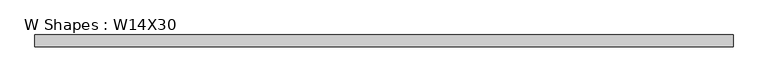
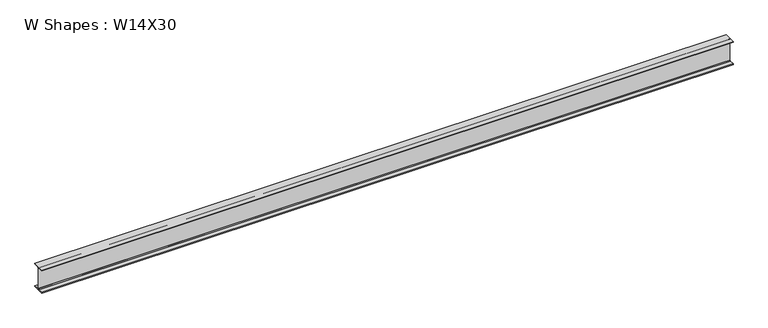
"""IFC4 building model written with IfcOpenShell, lengths in millimetres: beam geometry, W Shapes : W14X30."""

from ifc_helpers import new_model, si_unit, point, frame, frame_2d, origin, place, context, project, spatial, polyline, circle_curve, trimmed, segment, composite_curve, outline, extrude, source, transform, mapped, element, save


def w_shapes_w14x30_541e514d(model_context):
    return source(origin(), model_context, "Body", "SweptSolid", [
        extrude(outline(composite_curve([segment(polyline([(85.471, -165.481), (85.471, -175.26), (-85.471, -175.26), (-85.471, -165.481), (-13.589, -165.481)]), True, "CONTINUOUS"), segment(trimmed(circle_curve(frame_2d((-13.589, -155.321)), 10.16), [point((-13.589, -165.481))], [point((-3.429, -155.321))], True, "CARTESIAN"), True, "CONTINUOUS"), segment(polyline([(-3.429, -155.321), (-3.429, 155.321)]), True, "CONTINUOUS"), segment(trimmed(circle_curve(frame_2d((-13.589, 155.321)), 10.16), [point((-3.429, 155.321))], [point((-13.589, 165.481))], True, "CARTESIAN"), True, "CONTINUOUS"), segment(polyline([(-13.589, 165.481), (-85.471, 165.481), (-85.471, 175.26), (85.471, 175.26), (85.471, 165.481), (13.589, 165.481)]), True, "CONTINUOUS"), segment(trimmed(circle_curve(frame_2d((13.589, 155.321)), 10.16), [point((13.589, 165.481))], [point((3.429, 155.321))], True, "CARTESIAN"), True, "CONTINUOUS"), segment(polyline([(3.429, 155.321), (3.429, -155.321)]), True, "CONTINUOUS"), segment(trimmed(circle_curve(frame_2d((13.589, -155.321)), 10.16), [point((3.429, -155.321))], [point((13.589, -165.481))], True, "CARTESIAN"), True, "CONTINUOUS"), segment(polyline([(13.589, -165.481), (85.471, -165.481)]), True, "CONTINUOUS")], self_intersect=False)), frame((-5000.0, 0.0, 0.0), z_axis=(1.0, 0.0, 0.0), x_axis=(0.0, 1.0, 0.0)), (0.0, 0.0, 1.0), 10000.0),
    ])


if __name__ == "__main__":
    model = new_model("IFC4")
    model_context = context("Model", 3, world=origin())
    ifc_project = project(units=[si_unit("LENGTHUNIT", "METRE", prefix="MILLI")], contexts=[model_context])
    site = spatial("IfcSite", under=ifc_project)
    building = spatial("IfcBuilding", under=site)
    placement = place(None, origin())
    w_shapes_w14x30_shape = w_shapes_w14x30_541e514d(model_context)
    element("IfcBeam", 1, ObjectType="W Shapes : W14X30", at=placement, inside=building, context=model_context, shape_type="MappedRepresentation", body=[
        mapped(w_shapes_w14x30_shape, transform((0.0, 0.0, 0.0), x_axis=(1.0, 0.0, 0.0), y_axis=(0.0, 1.0, 0.0), z_axis=(0.0, 0.0, 1.0))),
    ])
    save(model, "model.ifc")

# Revit data of these elements
# Type "W Shapes : W14X30"
#   Section Name Key = "W14X30"
#   Width = 6.730"
#   Web Thickness = 0.270"
#   Web Fillet = 0.400"
#   Warping Constant = 887.00 in⁶
#   Torsional Moment of Inertia = 0.38 in⁴
#   Section Area = 8.85 in²
#   Plastic Modulus weak axis = 8.99 in³
#   Plastic Modulus strong axis = 47.30 in³
#   Perimeter = 4.441 ft²/ft
#   Nominal Weight = 30.00 lbf/ft
#   Moment of Inertia weak axis = 19.60 in⁴
#   Moment of Inertia strong axis = 291.00 in⁴
#   Height = 13.800"
#   Flange Thickness = 0.385"
#   Elastic Modulus weak axis = 5.82 in³
#   Elastic Modulus strong axis = 42.00 in³
#   Clear Web Height = 0' - 11 5/8"
#   Centroid Vertical = 6.900"
#   Centroid Horizontal = 3.365"
#   Bolt Spacing = 0' - 3 1/2"
#   Length [instance default] = 1524 mm
#   Structural Material [instance default] = Steel ASTM A992
#   Principal Axes Angle = 0
# Element 1 (IfcBeam, "W Shapes : W14X30")
#   Length = 5000 mm
#   Materials on its faces: "Steel ASTM A992"
# Materials
#   "Steel ASTM A992": class "Metal", colour RGB 199 199 199, transparency 0, Description = "Structural steel 50ksi", Cost = 0
